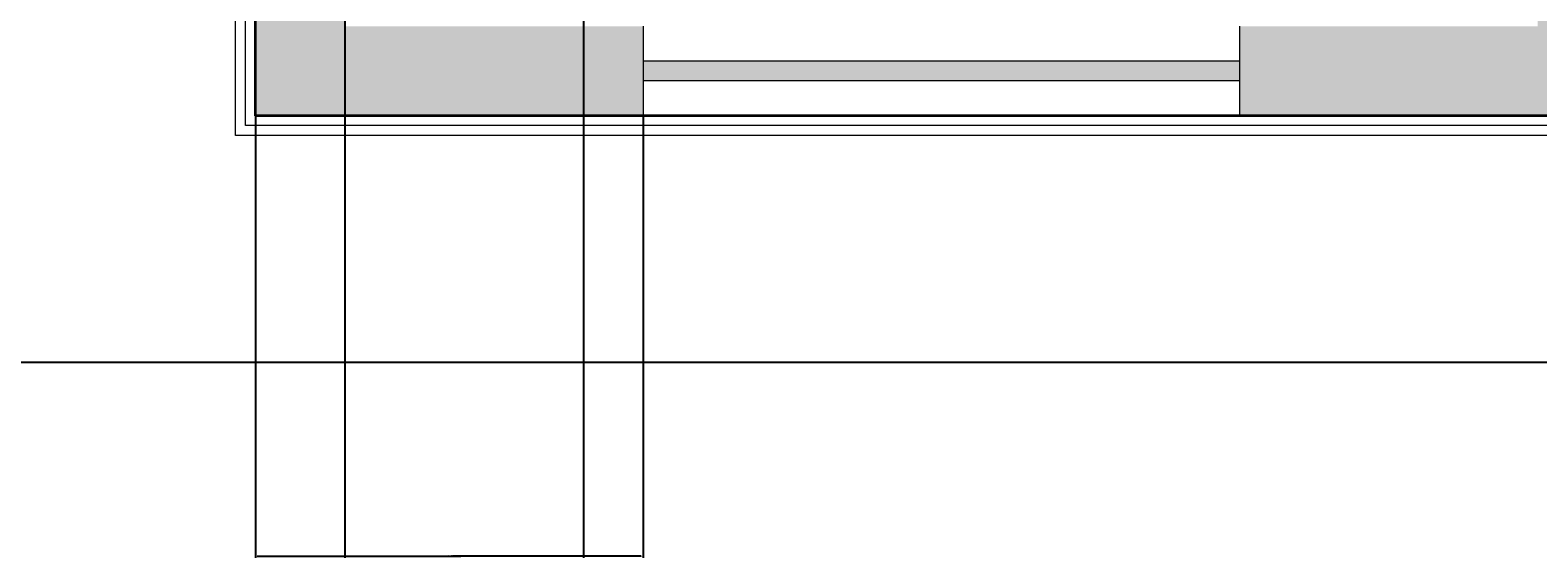
# Model space of a CAD drawing. Units: inches. Extents: x 311 to 815, y -527 to 136.
# Tile 2 of 21: x 388 to 539, y -527 to -474. Entities that reach past the tile are written whole.
import ezdxf

# ---------------------------------------------------------------- set-up
doc = ezdxf.new("R2010")
doc.units = ezdxf.units.IN
doc.header["$MEASUREMENT"] = 0
for name, color, linetype, lineweight in [('A-ANNO-DIMS', 1, 'Continuous', 18), ('A-ANNO-TTLB', 1, 'Continuous', 25), ('A-FLOR-EDGE', 1, 'Continuous', 18), ('A-GLAZ-PATT', 5, 'Continuous', 13), ('A-WALL-PATT', 242, 'Continuous', 13), ('wall', 1, 'Continuous', 35), ('win', 5, 'Continuous', 18)]:
    doc.layers.add(name, color=color, linetype=linetype, lineweight=lineweight)
doc.styles.get("Standard").update_dxf_attribs({"font": 'arial.ttf'})
doc.dimstyles.get("Standard").update_dxf_attribs({"dimtxt": 0.18, "dimasz": 0.18, "dimexe": 0.18, "dimexo": 0.0625, "dimgap": 0.09, "dimtad": 0, "dimtih": 1, "dimtoh": 1, "dimdec": 1, "dimzin": 0, "dimdsep": 46, "dimlunit": 4, "dimtxsty": 'Standard', "dimcen": 0.09, "dimadec": 0, "dimazin": 0, "dimtfac": 1, "dimtdec": 1, "dimtofl": 0, "dimtmove": 0, "dimatfit": 3, "dimfxl": 1, "dimtolj": 1, "dimtzin": 0, "dimarcsym": 0})

# ---------------------------------------------------------------- blocks, each defined once
blk = doc.blocks.new('_ArchTick')
at = {"color": 0, "linetype": 'ByBlock', "const_width": 0.15}
blk.add_lwpolyline([(-0.5, -0.5), (0.5, 0.5)], dxfattribs=at)
blk = doc.blocks.new('_Oblique')
at = {"color": 0, "linetype": 'ByBlock', "lineweight": -2}
blk.add_line((-0.5, -0.5), (0.5, 0.5), dxfattribs=at)
blk = doc.blocks.new('*D3')
at = {"layer": 'A-ANNO-DIMS', "color": 0, "lineweight": -2, "transparency": 16777216}
for p, q in [((377.54, 21.87), (377.54, -221.61)), ((377.54, -482.13), (377.54, -238.65))]:
    blk.add_line(p, q, dxfattribs=at)
at = {"layer": 'Defpoints', "color": 0, "transparency": 16777216}
for p in [(410.32, 21.87), (377.54, -482.13), (410.32, -482.13)]:
    blk.add_point(p, dxfattribs=at)
at = {"layer": 'A-ANNO-DIMS', "color": 0, "lineweight": -2, "transparency": 16777216, "xscale": 9, "yscale": 9, "zscale": 9}
for name, p, rotation in [('_ArchTick', (377.54, 21.87), 90), ('_Oblique', (377.54, -482.13), 270)]:
    blk.add_blockref(name, p, dxfattribs=dict(at, rotation=rotation))
at = {"layer": 'A-ANNO-DIMS', "color": 0, "transparency": 16777216, "insert": (377.54, -230.13), "char_height": 9, "attachment_point": 5}
blk.add_mtext("\\A1;42'", dxfattribs=at)
blk = doc.blocks.new('WIN-60IN')
for p, q in [((9, 60), (0, 60)), ((3.5, 0), (3.5, 60)), ((5.5, 0), (5.5, 60)), ((9, 0), (0, 0))]:
    blk.add_line(p, q)
blk = doc.blocks.new('*D26')
at = {"layer": 'A-ANNO-DIMS', "color": 0, "lineweight": -2, "transparency": 16777216}
for p, q in [((410.32, -482.19), (410.32, -526.66)), ((449.32, -482.19), (449.32, -526.66)), ((410.5, -526.48), (429.49, -526.48)), ((449.14, -526.48), (430.15, -526.48))]:
    blk.add_line(p, q, dxfattribs=at)
at = {"layer": 'A-ANNO-DIMS', "color": 0, "transparency": 16777216}
for points in [[(410.5, -526.45), (410.5, -526.51), (410.32, -526.48)], [(449.14, -526.45), (449.14, -526.51), (449.32, -526.48)]]:
    blk.add_solid(points, dxfattribs=at)
at = {"layer": 'Defpoints', "color": 0, "transparency": 16777216}
for p in [(410.32, -482.13), (449.32, -482.13), (449.32, -526.48)]:
    blk.add_point(p, dxfattribs=at)
at = {"layer": 'A-ANNO-DIMS', "color": 0, "transparency": 16777216, "insert": (429.82, -526.48), "char_height": 0.18, "attachment_point": 5}
blk.add_mtext('\\A1;3\'-3"', dxfattribs=at)
blk = doc.blocks.new('*D54')
at = {"layer": 'A-ANNO-DIMS', "color": 0, "lineweight": -2, "transparency": 16777216}
for p, q in [((419.32, -335.63), (419.32, -526.66)), ((443.32, -348.19), (443.32, -526.66)), ((419.5, -526.48), (430.99, -526.48)), ((443.14, -526.48), (431.65, -526.48))]:
    blk.add_line(p, q, dxfattribs=at)
at = {"layer": 'A-ANNO-DIMS', "color": 0, "transparency": 16777216}
for points in [[(419.5, -526.45), (419.5, -526.51), (419.32, -526.48)], [(443.14, -526.45), (443.14, -526.51), (443.32, -526.48)]]:
    blk.add_solid(points, dxfattribs=at)
at = {"layer": 'Defpoints', "color": 0, "transparency": 16777216}
for p in [(419.32, -335.57), (443.32, -348.13), (443.32, -526.48)]:
    blk.add_point(p, dxfattribs=at)
at = {"layer": 'A-ANNO-DIMS', "color": 0, "transparency": 16777216, "insert": (431.32, -526.48), "char_height": 0.18, "attachment_point": 5}
blk.add_mtext('\\A1;2\'-0"', dxfattribs=at)

msp = doc.modelspace()

# ---------------------------------------------------------------- hatches: boundary and pattern name
at = {"layer": 'A-GLAZ-PATT'}
h = msp.add_hatch(color=256, dxfattribs=at)
h.dxf.hatch_style = 1
h.paths.add_polyline_path([(415.82, -202.13), (413.82, -202.13), (413.82, -262.13), (415.82, -262.13)])
h.paths.add_polyline_path([(415.82, -390.84), (413.82, -390.84), (413.82, -450.84), (415.82, -450.84)])
h.paths.add_polyline_path([(415.82, -311.57), (413.82, -311.57), (413.82, -335.57), (415.82, -335.57)])
h.paths.add_polyline_path([(509.32, -476.63), (449.32, -476.63), (449.32, -478.63), (509.32, -478.63)])
h.paths.add_polyline_path([(606.82, -476.63), (582.82, -476.63), (582.82, -478.63), (606.82, -478.63)])
h.paths.add_polyline_path([(678.82, -476.63), (654.82, -476.63), (654.82, -478.63), (678.82, -478.63)])
h.paths.add_polyline_path([(718.82, -385.13), (716.82, -385.13), (716.82, -445.13), (718.82, -445.13)])
h.paths.add_polyline_path([(718.82, -262.63), (716.82, -262.63), (716.82, -322.63), (718.82, -322.63)])
h.paths.add_polyline_path([(718.82, -140.13), (716.82, -140.13), (716.82, -200.13), (718.82, -200.13)])
h.paths.add_polyline_path([(718.82, -18.13), (716.82, -18.13), (716.82, -42.13), (718.82, -42.13)])
h.paths.add_polyline_path([(686.82, 18.37), (626.82, 18.37), (626.82, 16.37), (686.82, 16.37)])
h.paths.add_polyline_path([(581.82, 18.37), (557.82, 18.37), (557.82, 16.37), (581.82, 16.37)])
h.paths.add_polyline_path([(509.32, 18.37), (449.32, 18.37), (449.32, 16.37), (509.32, 16.37)])
at = {"layer": 'A-WALL-PATT'}
h = msp.add_hatch(color=256, dxfattribs=at)
h.dxf.hatch_style = 1
h.paths.add_polyline_path([(557.82, 21.87), (509.32, 21.87), (509.32, 12.87), (539.32, 12.87), (539.32, -112.13), (548.32, -112.13), (548.32, -58.63), (557.82, -58.63), (557.82, -49.63), (548.32, -49.63), (548.32, 12.87), (557.82, 12.87)])
h.paths.add_polyline_path([(449.32, 21.87), (410.32, 21.87), (410.32, -15.13), (419.32, -15.13), (419.32, 12.87), (449.32, 12.87)])
h.paths.add_polyline_path([(626.82, 21.87), (581.82, 21.87), (581.82, 12.87), (591.32, 12.87), (591.32, -49.63), (581.82, -49.63), (581.82, -58.63), (591.32, -58.63), (591.32, -112.13), (600.32, -112.13), (600.32, 12.87), (626.82, 12.87)])
h.paths.add_polyline_path([(722.32, 21.87), (686.82, 21.87), (686.82, 12.87), (713.32, 12.87), (713.32, -18.13), (722.32, -18.13)])
h.paths.add_polyline_path([(722.32, -42.13), (713.32, -42.13), (713.32, -73.13), (722.32, -73.13)])
h.paths.add_polyline_path([(501.32, -103.13), (419.32, -103.13), (419.32, -75.13), (410.32, -75.13), (410.32, -126.63), (419.32, -126.63), (419.32, -112.13), (492.32, -112.13), (492.32, -143.13), (501.32, -143.13)])
h.paths.add_polyline_path([(548.32, -165.13), (419.32, -165.13), (419.32, -150.63), (410.32, -150.63), (410.32, -202.13), (419.32, -202.13), (419.32, -174.13), (548.32, -174.13)])
h.paths.add_polyline_path([(722.32, -103.13), (636.32, -103.13), (636.32, -112.13), (713.32, -112.13), (713.32, -140.13), (722.32, -140.13)])
h.paths.add_polyline_path([(548.32, -210.13), (539.32, -210.13), (539.32, -290.13), (419.32, -290.13), (419.32, -262.13), (410.32, -262.13), (410.32, -311.57), (419.32, -311.57), (419.32, -299.13), (469.32, -299.13), (469.32, -348.13), (443.32, -348.13), (443.32, -357.13), (478.32, -357.13), (478.32, -299.13), (548.32, -299.13)])
h.paths.add_polyline_path([(722.32, -200.13), (713.32, -200.13), (713.32, -228.13), (609.32, -228.13), (609.32, -237.13), (713.32, -237.13), (713.32, -262.63), (722.32, -262.63)])
h.paths.add_polyline_path([(722.32, -322.63), (713.32, -322.63), (713.32, -348.13), (633.32, -348.13), (633.32, -357.13), (713.32, -357.13), (713.32, -385.13), (722.32, -385.13)])
h.paths.add_polyline_path([(419.32, -335.57), (410.32, -335.57), (410.32, -390.84), (419.32, -390.84)])
h.paths.add_polyline_path([(419.32, -450.84), (410.32, -450.84), (410.32, -482.13), (449.32, -482.13), (449.32, -473.13), (419.32, -473.13)])
h.paths.add_polyline_path([(582.82, -473.13), (548.32, -473.13), (548.32, -348.13), (539.32, -348.13), (539.32, -473.13), (509.32, -473.13), (509.32, -482.13), (582.82, -482.13)])
h.paths.add_polyline_path([(722.32, -445.13), (713.32, -445.13), (713.32, -473.13), (678.82, -473.13), (678.82, -482.13), (722.32, -482.13)])

# ---------------------------------------------------------------- linework, layer by layer
at = {"layer": 'A-ANNO-TTLB'}
msp.add_lwpolyline([(310.67, 136.01), (815.43, 136.01), (815.43, -506.97), (310.67, -506.97)], close=True, dxfattribs=at)
at = {"layer": 'A-FLOR-EDGE'}
for p, q in [((408.32, -484.13), (408.32, 23.87)), ((409.32, -483.13), (409.32, 22.87)), ((723.32, -483.13), (409.32, -483.13)), ((724.32, -484.13), (408.32, -484.13))]:
    msp.add_line(p, q, dxfattribs=at)
at = {"layer": 'wall'}
for p, q in [((410.32, -482.13), (410.32, 21.87)), ((722.32, -482.13), (410.32, -482.13))]:
    msp.add_line(p, q, dxfattribs=at)

# ---------------------------------------------------------------- block references
at = {"layer": 'win', "rotation": 90.00000000000003}
msp.add_blockref('WIN-60IN', (509.32, -482.13), dxfattribs=at)

# ---------------------------------------------------------------- dimensions: what is measured, and where the dimension line sits
at = {"layer": 'A-ANNO-DIMS'}
dim = msp.add_linear_dim(base=(377.54, -482.13), p1=(410.32, 21.87), p2=(410.32, -482.13), angle=90, dimstyle='Standard', override={"dimtxt": 9, "dimasz": 9, "dimgap": 4, "dimblk1": 'ArchTick', "dimblk2": 'Oblique', "dimsah": 1, "dimse1": 1, "dimse2": 1, "dimclrd": 0, "dimclre": 0, "dimclrt": 0}, dxfattribs=at)
dim.commit()
dim.dimension.update_dxf_attribs({"geometry": '*D3', "text_midpoint": (377.54, -230.13)})
for base, p1, p2, picture, middle in [((443.32, -526.48), (419.32, -335.57), (443.32, -348.13), '*D54', (431.32, -526.48)), ((449.32, -526.48), (410.32, -482.13), (449.32, -482.13), '*D26', (429.82, -526.48))]:
    dim = msp.add_linear_dim(base=base, p1=p1, p2=p2, dimstyle='Standard', override={"dimdec": 1, "dimlfac": 1, "dimrnd": 0, "dimzin": 1, "dimdsep": 46, "dimlunit": 4, "dimfrac": 2}, dxfattribs=at)
    dim.commit()
    dim.dimension.update_dxf_attribs({"geometry": picture, "text_midpoint": middle})

doc.saveas('drawing.dxf')
